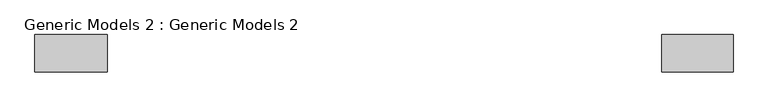
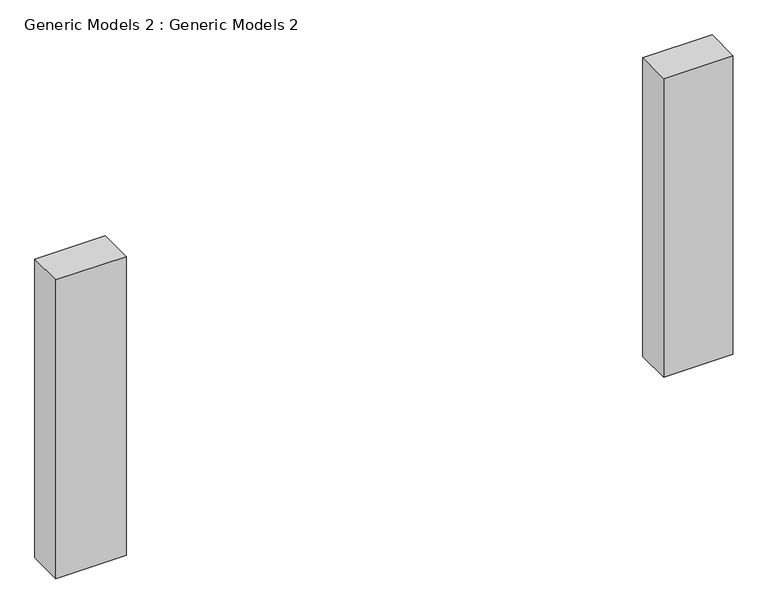
"""IFC4 building model written with IfcOpenShell, lengths in millimetres: proxy geometry, Generic Models 2 : Generic Models 2."""

from ifc_helpers import new_model, si_unit, origin, origin_with_axes, place, context, project, spatial, polyline, outline, extrude, source, transform, mapped, element, save


def generic_models_2_generic_models_2_43715522(model_context):
    return source(origin(), model_context, "Body", "SweptSolid", [
        extrude(outline(polyline([(-562.0138036, -3746.0004242), (-562.0138036, -4109.1187941), (-1266.3806312, -4109.1187941), (-1266.3806312, -3746.0004242), (-562.0138036, -3746.0004242)])), origin_with_axes(), (0.0, 0.0, 1.0), 3160.1299346),
        extrude(outline(polyline([(5509.6940308, -3746.0004242), (5509.6940308, -4107.3695548), (4815.8764826, -4107.3695548), (4815.8764826, -3746.0004242), (5509.6940308, -3746.0004242)])), origin_with_axes(), (0.0, 0.0, 1.0), 3160.1299346),
    ])


if __name__ == "__main__":
    model = new_model("IFC4")
    model_context = context("Model", 3, world=origin())
    ifc_project = project(units=[si_unit("LENGTHUNIT", "METRE", prefix="MILLI")], contexts=[model_context])
    site = spatial("IfcSite", under=ifc_project)
    building = spatial("IfcBuilding", under=site)
    placement = place(None, origin())
    generic_models_2_generic_models_2_shape = generic_models_2_generic_models_2_43715522(model_context)
    element("IfcBuildingElementProxy", 1, Name="Generic Models 2 : Generic Models 2", ObjectType="Generic Models 2 : Generic Models 2", at=placement, inside=building, context=model_context, shape_type="MappedRepresentation", body=[
        mapped(generic_models_2_generic_models_2_shape, transform((0.0, 0.0, 0.0), x_axis=(1.0, 0.0, 0.0), y_axis=(0.0, 1.0, 0.0), z_axis=(0.0, 0.0, 1.0))),
    ])
    save(model, "model.ifc")
